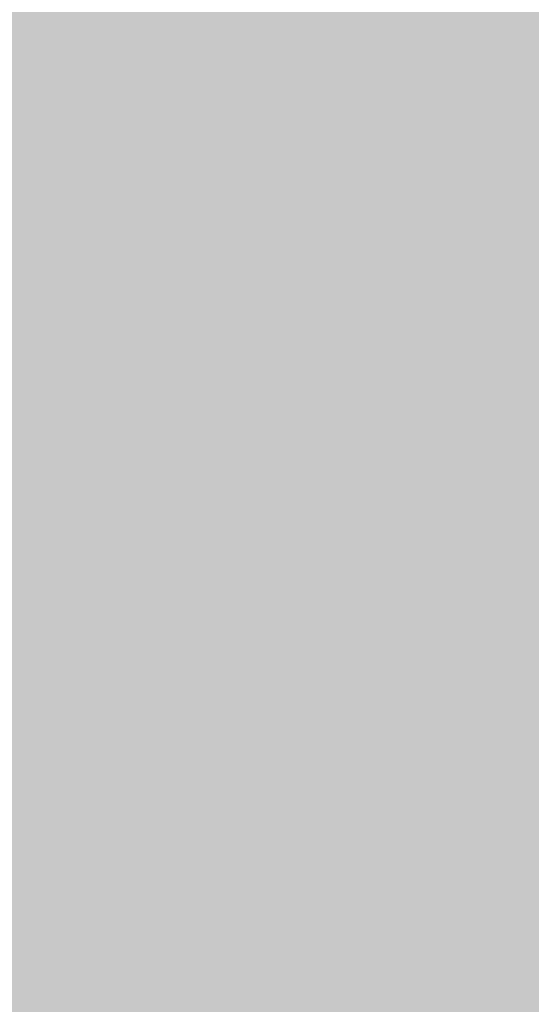
# Model space of a CAD drawing. Units: inches. Extents: x 2083 to 3317, y 1141 to 2115.
# Tile 206 of 256: x 3126.132 to 3126.67, y 1264.131 to 1265.165. Entities that reach past the tile are written whole.
import ezdxf

# ---------------------------------------------------------------- set-up
doc = ezdxf.new("R2010")
doc.units = ezdxf.units.IN
doc.layers.add('A-ANNO-DIMS', color=2, linetype='Continuous', lineweight=18)
doc.layers.add('A-WALL-PATT', color=251, linetype='Continuous', lineweight=13, true_color=0x636466)
doc.styles.get("Standard").update_dxf_attribs({"font": 'arial.ttf'})
doc.dimstyles.new('ISO-25', dxfattribs={"dimtxt": 12, "dimasz": 12, "dimexe": 1.25, "dimexo": 0.625, "dimtad": 1, "dimlunit": 3, "dimtxsty": 'Standard', "dimcen": 2.5, "dimadec": 0, "dimazin": 0, "dimtfac": 1, "dimtmove": 0, "dimatfit": 3, "dimfxl": 1, "dimarcsym": 0})

# ---------------------------------------------------------------- blocks, each defined once
blk = doc.blocks.new('*D26')
at = {"layer": 'A-ANNO-DIMS', "color": 0, "lineweight": -2, "transparency": 16777216}
for p, q in [((3088.9858, 1274.9151), (3088.9858, 1270.952)), ((3111.24, 1274.9151), (3111.24, 1270.952)), ((3076.9858, 1272.202), (2840.2624, 1272.202)), ((3111.24, 1272.202), (3088.9858, 1272.202)), ((3123.24, 1272.202), (3135.24, 1272.202))]:
    blk.add_line(p, q, dxfattribs=at)
at = {"layer": 'A-ANNO-DIMS', "color": 0, "transparency": 16777216}
for points in [[(3076.9858, 1274.202), (3076.9858, 1270.202), (3088.9858, 1272.202)], [(3123.24, 1274.202), (3123.24, 1270.202), (3111.24, 1272.202)]]:
    blk.add_solid(points, dxfattribs=at)
at = {"layer": 'Defpoints', "color": 0, "transparency": 16777216}
for p in [(3088.9858, 1275.5401), (3111.24, 1275.5401), (3088.9858, 1272.202)]:
    blk.add_point(p, dxfattribs=at)
at = {"layer": 'A-ANNO-DIMS', "color": 0, "transparency": 16777216, "insert": (2952.6241, 1279.0316), "char_height": 12, "attachment_point": 5}
blk.add_mtext('NIGHTSTAND 1\'-10 1/2" TYP.', dxfattribs=at)
blk = doc.blocks.new('*D27')
at = {"layer": 'A-ANNO-DIMS', "color": 0, "lineweight": -2, "transparency": 16777216}
for p, q in [((3114.5782, 1309.7943), (3114.5782, 1321.7943)), ((3111.865, 1297.7943), (3115.8282, 1297.7943)), ((3114.5782, 1297.7943), (3114.5782, 1275.5401)), ((3111.865, 1275.5401), (3115.8282, 1275.5401)), ((3114.5782, 1263.5401), (3114.5782, 1140.9886))]:
    blk.add_line(p, q, dxfattribs=at)
at = {"layer": 'A-ANNO-DIMS', "color": 0, "transparency": 16777216}
for points in [[(3112.5782, 1309.7943), (3116.5782, 1309.7943), (3114.5782, 1297.7943)], [(3112.5782, 1263.5401), (3116.5782, 1263.5401), (3114.5782, 1275.5401)]]:
    blk.add_solid(points, dxfattribs=at)
at = {"layer": 'Defpoints', "color": 0, "transparency": 16777216}
for p in [(3111.24, 1297.7943), (3111.24, 1275.5401), (3114.5782, 1275.5401)]:
    blk.add_point(p, dxfattribs=at)
at = {"layer": 'A-ANNO-DIMS', "color": 0, "transparency": 16777216, "insert": (3107.7485, 1196.2643), "char_height": 12, "attachment_point": 5, "rotation": 90}
blk.add_mtext('1\'-10 1/2" TYP.', dxfattribs=at)

msp = doc.modelspace()

# ---------------------------------------------------------------- hatches: boundary and pattern name
at = {"layer": 'A-WALL-PATT'}
h = msp.add_hatch(color=256, dxfattribs=at)
h.dxf.hatch_style = 1
h.paths.add_polyline_path([(3126.9598, 2020.7614), (2748.9598, 2020.7614), (2604.9598, 2020.7614), (2226.9598, 2020.7614), (2226.9598, 1702.7614), (2466.9598, 1702.7614), (2466.9598, 1582.7614), (2418.9598, 1582.7614), (2418.9598, 1477.7614), (2226.9598, 1477.7614), (2226.9598, 1263.2614), (2544.9598, 1263.2614), (2544.9598, 1411.7614), (2604.9598, 1411.7614), (2685.9598, 1411.7614), (2685.9598, 1420.7614), (2604.9598, 1420.7614), (2604.9598, 1573.7614), (2604.9598, 1702.7614), (2604.9598, 2011.7614), (2748.9598, 2011.7614), (2748.9598, 1702.7614), (2862.9598, 1702.7614), (2862.9598, 1621.7614), (2871.9598, 1621.7614), (2871.9598, 1702.7614), (2883.9598, 1702.7614), (2883.9598, 1706.9395, -0.026459), (2883.9598, 1711.7614), (2757.9598, 1711.7614), (2757.9598, 1807.7614), (2787.9598, 1807.7614), (2787.9598, 1812.2614), (2757.9598, 1812.2614), (2757.9598, 2011.7614), (2877.9598, 2011.7614), (2877.9598, 1812.2614), (2847.9598, 1812.2614), (2847.9598, 1807.7614), (2889.8357, 1807.7614), (2889.8357, 1812.2614), (2882.4598, 1812.2614), (2882.4598, 2011.7614), (3117.9598, 2011.7614), (3117.9598, 1812.2614), (2937.8357, 1812.2614), (2937.8357, 1807.7614), (2995.7098, 1807.7614), (2995.7098, 1796.1177), (3000.2098, 1796.1177), (3000.2098, 1807.7614), (3117.9598, 1807.7614), (3117.9598, 1711.7614), (3000.2098, 1711.7614), (3000.2098, 1760.1177), (2998.5727, 1760.1177, -0.020711), (2995.7098, 1760.1177), (2995.7098, 1711.7614), (2931.9598, 1711.7614), (2931.9598, 1702.7614), (3126.9598, 1702.7614)])
h.paths.add_polyline_path([(2471.4598, 2011.7614), (2471.4598, 1810.0114), (2462.7169, 1810.0114), (2462.7169, 1805.5114), (2505.9598, 1805.5114), (2505.9598, 1810.0114), (2475.9598, 1810.0114), (2475.9598, 2011.7614), (2595.9598, 2011.7614), (2595.9598, 1810.0114), (2565.9598, 1810.0114), (2565.9598, 1805.5114), (2595.9598, 1805.5114), (2595.9598, 1711.7614), (2235.9598, 1711.7614), (2235.9598, 1805.5114), (2353.7098, 1805.5114), (2353.7098, 1796.0542), (2358.2098, 1796.0542), (2358.2098, 1805.5114), (2414.7169, 1805.5114), (2414.7169, 1810.0114), (2235.9598, 1810.0114), (2235.9598, 2011.7614)], flags=16)
h.paths.add_polyline_path([(2270.2047, 1994.61), (2270.2047, 1970.61), (2246.2047, 1970.61), (2246.2047, 1994.61)], flags=0)
edge = h.paths.add_edge_path(flags=0)
edge.add_ellipse((2332.0274, 1899.7982), major_axis=(-3.043, 3.043), ratio=0.168252, start_angle=-161.3322, end_angle=-156.3071, ccw=False)
edge.add_ellipse((2333.082, 1898.7435), major_axis=(-1.0546, 1.0546), ratio=0.453532, start_angle=-123.371, end_angle=-94.1591)
edge = h.paths.add_edge_path(flags=0)
edge.add_ellipse((2332.0274, 1968.8763), major_axis=(3.043, 3.043), ratio=0.168252, start_angle=18.6678, end_angle=23.6929)
edge.add_spline(control_points=[(2332.9256, 1970.6911), (2332.2268, 1970.3361), (2330.8937, 1969.6589), (2328.4131, 1970.9321), (2327.2039, 1967.7487), (2324.7096, 1969.9556), (2322.5328, 1967.0124), (2320.0128, 1971.2958), (2317.6803, 1968.1578), (2316.0405, 1967.102), (2315.4269, 1966.8096)], knot_values=[0, 0, 0, 0, 2.267059, 4.324559, 6.685584, 8.878641, 11.121502, 14.300359, 17.755284, 19.732645, 19.732645, 19.732645, 19.732645], degree=3, periodic=0)
edge.add_ellipse((2332.0274, 1968.8763), major_axis=(3.043, 3.043), ratio=0.168252, start_angle=18.6678, end_angle=23.6929, ccw=False)
edge.add_ellipse((2333.082, 1969.9309), major_axis=(1.0546, 1.0546), ratio=0.453532, start_angle=56.629, end_angle=85.8409, ccw=False)
edge = h.paths.add_edge_path(flags=0)
edge.add_spline(control_points=[(2296.4283, 1967.9879), (2293.6278, 1965.3363), (2287.7036, 1959.7271), (2299.7439, 1949.9957), (2294.5326, 1935.6685), (2290.5732, 1920.6035), (2293.3941, 1909.9737), (2296.1854, 1904.9665)], knot_values=[0.099185, 0.099185, 0.099185, 0.099185, 0.345301, 0.619822, 0.982653, 1.386093, 1.810555, 1.810555, 1.810555, 1.810555], degree=3, periodic=0)
edge.add_spline(control_points=[(2296.1854, 1904.9665), (2297.3836, 1902.6193), (2298.001, 1901.9493), (2298.553, 1901.4682)], knot_values=[0.006246, 0.006246, 0.006246, 0.006246, 0.055476, 0.055476, 0.055476, 0.055476], degree=3, periodic=0)
edge.add_spline(control_points=[(2298.553, 1901.4682), (2297.2586, 1900.9232), (2295.2253, 1900.2321), (2293.0602, 1900.6142), (2292.1014, 1900.7884), (2292.0896, 1900.7906)], knot_values=[0.312835, 0.312835, 0.312835, 0.312835, 0.40178, 0.474987, 0.475903, 0.475903, 0.475903, 0.475903], degree=3, periodic=0)
edge.add_arc((2292.7936, 1904.6641), 3.937, 215.4209, 259.6982, ccw=False)
edge.add_spline(control_points=[(2289.5853, 1902.3823), (2289.4767, 1902.5351), (2289.3685, 1902.688), (2289.2609, 1902.8412)], knot_values=[0.102872, 0.102872, 0.102872, 0.102872, 0.116896, 0.116896, 0.116896, 0.116896], degree=3, periodic=0)
edge.add_spline(control_points=[(2289.2609, 1902.8412), (2288.6866, 1902.5502), (2287.64, 1902.0199), (2285.8813, 1901.874), (2283.853, 1901.5044), (2281.72, 1899.7105), (2278.467, 1899.4929), (2276.1571, 1901.8832), (2272.259, 1899.8041), (2267.7776, 1901.8432), (2262.2439, 1900.184), (2257.4149, 1901.7821), (2254.3184, 1900.7261), (2253.1783, 1900.3373)], knot_values=[0, 0, 0, 0, 1.907977, 3.477176, 5.261074, 7.972851, 11.680248, 13.717921, 16.939592, 22.789562, 27.502503, 33.595215, 37.145618, 37.145618, 37.145618, 37.145618], degree=3, periodic=0)
edge.add_line((2253.1783, 1900.3373), (2250.2442, 1902.8412))
edge.add_line((2250.2442, 1902.8412), (2250.2442, 1965.8333))
edge.add_line((2250.2442, 1965.8333), (2253.1783, 1968.3371))
edge.add_spline(control_points=[(2253.1783, 1968.3371), (2254.3184, 1967.9483), (2257.4149, 1966.8924), (2262.2439, 1968.4904), (2267.7776, 1966.8313), (2271.5267, 1968.5372), (2273.8759, 1967.8283), (2274.2067, 1967.7276)], knot_values=[0, 0, 0, 0, 0.09018, 0.244935, 0.364644, 0.513233, 0.537855, 0.537855, 0.537855, 0.537855], degree=3, periodic=0)
edge.add_arc((2274.3529, 1963.7933), 3.937, 72.0511, 92.1279, ccw=False)
edge.add_arc((2281.2969, 1985.23), 18.5963, 252.05113, 288.56572)
edge.add_arc((2292.3167, 1956.0289), 12.6461, 71.02679, 113.77822, ccw=False)
edge = h.paths.add_edge_path(flags=0)
edge.add_spline(control_points=[(2274.8994, 1951.8562), (2275.0662, 1951.6166), (2275.2327, 1951.3766), (2275.398, 1951.1359)], knot_values=[1.409916, 1.409916, 1.409916, 1.409916, 1.43159, 1.43159, 1.43159, 1.43159], degree=3, periodic=0)
edge.add_spline(control_points=[(2275.398, 1951.1359), (2275.7921, 1950.5619), (2276.1792, 1949.9838), (2276.5455, 1949.3971)], knot_values=[1.358238, 1.358238, 1.358238, 1.358238, 1.409916, 1.409916, 1.409916, 1.409916], degree=3, periodic=0)
edge.add_line((2276.5455, 1949.3971), (2277.4373, 1947.8622))
edge.add_spline(control_points=[(2277.4373, 1947.8622), (2276.3038, 1945.6731), (2274.6397, 1942.4269), (2274.6316, 1938.0939), (2272.7991, 1930.8515), (2274.3564, 1943.897), (2275.9477, 1947.9234), (2276.5455, 1949.3971)], knot_values=[0.005632, 0.005632, 0.005632, 0.005632, 0.186014, 0.266002, 0.357087, 0.59639, 0.739732, 0.739732, 0.739732, 0.739732], degree=3, periodic=0)
edge.add_spline(control_points=[(2276.5455, 1949.3971), (2276.1792, 1949.9838), (2275.7921, 1950.5619), (2275.398, 1951.1359)], knot_values=[1.358238, 1.358238, 1.358238, 1.358238, 1.409916, 1.409916, 1.409916, 1.409916], degree=3, periodic=0)
edge.add_spline(control_points=[(2275.398, 1951.1359), (2274.9425, 1950.0805), (2274.2078, 1948.0253), (2273.9346, 1944.8515), (2272.4685, 1937.6275), (2273.4662, 1945.6965), (2274.7006, 1951.0595), (2274.8994, 1951.8562)], knot_values=[0.104364, 0.104364, 0.104364, 0.104364, 0.189636, 0.269624, 0.36071, 0.600013, 0.644622, 0.644622, 0.644622, 0.644622], degree=3, periodic=0)
h.paths.add_polyline_path([(2269.1675, 1963.1276, -0.357527), (2268.1706, 1960.9764, -0.092561), (2268.1706, 1939.4363, -0.357527), (2269.1675, 1937.2851, -0.357527), (2267.0163, 1938.282, -0.164785), (2254.6856, 1938.282, -0.357527), (2252.5344, 1937.2851, -0.357527), (2253.5313, 1939.4363, -0.092561), (2253.5313, 1960.9764, -0.357527), (2252.5344, 1963.1276, -0.357527), (2254.6856, 1962.1307, -0.164785), (2267.0163, 1962.1307, -0.357527)], flags=0)
h.paths.add_polyline_path([(2248.8741, 1967.8018), (2248.8741, 1957.0277), (2249.4578, 1957.0277), (2249.4578, 1911.6468), (2248.8741, 1911.6468), (2248.8741, 1900.8727), (2246.5119, 1900.8727, 0.197327), (2244.1497, 1902.4569), (2244.1497, 1966.2176, 0.197327), (2246.5119, 1967.8018)], flags=0)
h.paths.add_polyline_path([(2269.1675, 1931.3893, -0.357527), (2268.1706, 1929.2381, -0.092561), (2268.1706, 1907.6981, -0.357527), (2269.1675, 1905.5469, -0.357527), (2267.0163, 1906.5438, -0.164785), (2254.6856, 1906.5438, -0.357527), (2252.5344, 1905.5469, -0.357527), (2253.5313, 1907.6981, -0.092561), (2253.5313, 1929.2381, -0.357527), (2252.5344, 1931.3893, -0.357527), (2254.6856, 1930.3925, -0.164785), (2267.0163, 1930.3925, -0.357527)], flags=0)
edge = h.paths.add_edge_path(flags=0)
edge.add_spline(control_points=[(2276.1969, 1906.7237), (2276.1681, 1909.0289), (2276.114, 1913.3719), (2270.5984, 1924.925), (2273.9052, 1919.0128), (2275.9217, 1916.2621), (2275.4746, 1912.4021), (2277.2579, 1910.3806), (2276.696, 1908.225), (2276.6462, 1906.813), (2276.6178, 1906.0084)], knot_values=[0, 0, 0, 0, 8.61026, 16.221274, 18.843057, 23.804898, 27.440828, 29.356102, 31.203478, 33.650687, 33.650687, 33.650687, 33.650687], degree=3, periodic=0)
edge.add_spline(control_points=[(2276.6178, 1906.0084), (2276.6233, 1905.6241), (2276.4977, 1904.6287), (2275.4418, 1903.8547), (2274.9373, 1903.0804), (2274.8591, 1902.8412)], knot_values=[0.156488, 0.156488, 0.156488, 0.156488, 0.184398, 0.231376, 0.250598, 0.250598, 0.250598, 0.250598], degree=3, periodic=0)
edge.add_line((2274.8591, 1902.8412), (2276.506, 1902.8412))
edge.add_spline(control_points=[(2276.506, 1902.8412), (2276.7883, 1903.0849), (2277.6651, 1904.1252), (2278.2495, 1904.3407), (2277.6539, 1908.5274), (2278.1557, 1906.2278), (2278.1005, 1905.2859), (2278.8467, 1904.069), (2277.8568, 1903.4149), (2277.8742, 1902.991), (2277.9036, 1902.8412)], knot_values=[0.059574, 0.059574, 0.059574, 0.059574, 0.080753, 0.103741, 0.16972, 0.176036, 0.207137, 0.240474, 0.262341, 0.27366, 0.27366, 0.27366, 0.27366], degree=3, periodic=0)
edge.add_line((2277.9036, 1902.8412), (2280.0298, 1902.8412))
edge.add_spline(control_points=[(2280.0298, 1902.8412), (2279.8882, 1903.0884), (2279.4993, 1903.9816), (2280.1523, 1905.9393), (2278.1036, 1909.6578), (2279.7624, 1907.1853), (2280.3279, 1904.8749), (2280.4851, 1903.4896), (2281.4633, 1903.2494), (2281.7583, 1902.9365), (2281.834, 1902.8412)], knot_values=[0.013856, 0.013856, 0.013856, 0.013856, 0.034874, 0.088867, 0.107879, 0.126738, 0.158714, 0.193757, 0.217487, 0.226722, 0.226722, 0.226722, 0.226722], degree=3, periodic=0)
edge.add_spline(control_points=[(2281.834, 1902.8412), (2281.7875, 1902.8267), (2281.647, 1902.783), (2281.3955, 1902.8595), (2281.0881, 1902.9852), (2280.7207, 1903.0609), (2280.3335, 1903.0257), (2280.1248, 1902.8989), (2280.0298, 1902.8412)], knot_values=[0, 0, 0, 0, 0.14413, 0.435517, 0.749276, 1.153046, 1.548371, 1.878348, 1.878348, 1.878348, 1.878348], degree=3, periodic=0)
edge.add_line((2280.0298, 1902.8412), (2277.9036, 1902.8412))
edge.add_spline(control_points=[(2277.9036, 1902.8412), (2277.8929, 1902.7959), (2277.8654, 1902.6796), (2277.6075, 1902.6875), (2277.2741, 1902.8007), (2276.8379, 1902.6198), (2276.5838, 1902.7893), (2276.506, 1902.8412)], knot_values=[0, 0, 0, 0, 0.127189, 0.326199, 0.628009, 1.24357, 1.515331, 1.515331, 1.515331, 1.515331], degree=3, periodic=0)
edge.add_line((2276.506, 1902.8412), (2274.8591, 1902.8412))
edge.add_spline(control_points=[(2274.8591, 1902.8412), (2274.8144, 1902.8986), (2274.7251, 1903.0134), (2274.4935, 1903.119), (2274.2443, 1902.9605), (2273.9371, 1903.1849), (2273.614, 1902.9831), (2273.4083, 1902.883), (2273.3223, 1902.8412)], knot_values=[0, 0, 0, 0, 0.21843, 0.436957, 0.687977, 0.990379, 1.398396, 1.69185, 1.69185, 1.69185, 1.69185], degree=3, periodic=0)
edge.add_spline(control_points=[(2273.3223, 1902.8412), (2273.6167, 1903.4457), (2274.274, 1904.5383), (2276.0272, 1904.5737), (2276.207, 1906.5836), (2276.1969, 1906.7237)], knot_values=[0.012227, 0.012227, 0.012227, 0.012227, 0.059472, 0.106218, 0.134458, 0.134458, 0.134458, 0.134458], degree=3, periodic=0)
h.paths.add_polyline_path([(2270.7761, 1897.7898), (2270.7761, 1873.7898), (2246.7761, 1873.7898), (2246.7761, 1897.7898)], flags=0)
h.paths.add_polyline_path([(2353.7098, 1760.0051), (2353.7098, 1760.0542), (2358.2098, 1760.0542, -0.033729)], flags=0)
h.paths.add_polyline_path([(2321.8191, 1737.5292), (2341.9953, 1737.5292, -0.414214), (2343.2033, 1736.3212), (2343.2033, 1721.0206, -0.414214), (2341.9953, 1719.8127), (2321.8191, 1719.8127, -0.414214), (2320.6112, 1721.0206), (2320.6112, 1736.3212, -0.414214)], flags=0)
h.paths.add_polyline_path([(2324.235, 1736.3212), (2339.5794, 1736.3212, -0.414214), (2341.9953, 1733.9053), (2341.9953, 1725.4497, -0.414214), (2339.5794, 1723.0338), (2333.6806, 1723.0338), (2333.8453, 1722.0455, -0.870646), (2335.4254, 1721.8259, -0.767327), (2333.9227, 1721.4232), (2331.291, 1721.4232, -0.767327), (2329.7883, 1721.8259, -0.870646), (2331.3684, 1722.0455), (2331.5331, 1723.0338), (2324.235, 1723.0338, -0.414214), (2321.8191, 1725.4497), (2321.8191, 1733.9053, -0.414214)], flags=0)
h.paths.add_polyline_path([(2570.4838, 1928.6154), (2589.6838, 1928.6154), (2590.1688, 1928.6154), (2590.1688, 1904.9934), (2570.4838, 1904.9934)], flags=0)
h.paths.add_polyline_path([(2574.4473, 1927.2638, -1), (2572.8288, 1927.2638, -1)], flags=0)
h.paths.add_polyline_path([(2573.0899, 1926.9409), (2573.925, 1927.776), (2574.1477, 1927.5533), (2573.3126, 1926.7182)], flags=0)
h.paths.add_polyline_path([(2578.7791, 1919.7296, -1), (2571.5917, 1919.7296, -1)], flags=0)
h.paths.add_polyline_path([(2578.3854, 1919.7296, -1), (2571.9854, 1919.7296, -1)], flags=0)
h.paths.add_polyline_path([(2331.5958, 1729.4762, -1), (2333.618, 1729.4762, -1)], flags=0)
h.paths.add_polyline_path([(2578.0342, 1927.2638, -1), (2576.4157, 1927.2638, -1)], flags=0)
h.paths.add_polyline_path([(2576.6889, 1927.5311), (2576.9116, 1927.7538), (2577.7467, 1926.9186), (2577.524, 1926.6959)], flags=0)
h.paths.add_polyline_path([(2578.1391, 1909.8595, -1), (2572.2317, 1909.8595, -1)], flags=0)
h.paths.add_polyline_path([(2577.7454, 1909.8595, -1), (2572.6254, 1909.8595, -1)], flags=0)
h.paths.add_polyline_path([(2583.7977, 1927.2638, -1), (2582.1792, 1927.2638, -1)], flags=0)
h.paths.add_polyline_path([(2582.7186, 1927.7538), (2583.5538, 1926.9186), (2583.3311, 1926.6959), (2582.4959, 1927.5311)], flags=0)
h.paths.add_polyline_path([(2582.4959, 1927.5311), (2582.7186, 1927.7538), (2583.5538, 1926.9186), (2583.3311, 1926.6959)], flags=0)
h.paths.add_polyline_path([(2587.7391, 1920.5296, -1), (2581.8317, 1920.5296, -1)], flags=0)
h.paths.add_polyline_path([(2587.3454, 1920.5296, -1), (2582.2254, 1920.5296, -1)], flags=0)
h.paths.add_polyline_path([(2587.3846, 1927.2638, -1), (2585.7661, 1927.2638, -1)], flags=0)
h.paths.add_polyline_path([(2586.082, 1926.9802), (2586.9172, 1927.8154), (2587.1399, 1927.5927), (2586.3047, 1926.7575)], flags=0)
h.paths.add_polyline_path([(2588.3791, 1910.6595, -1), (2581.1917, 1910.6595, -1)], flags=0)
h.paths.add_polyline_path([(2587.9854, 1910.6595, -1), (2581.5854, 1910.6595, -1)], flags=0)
h.paths.add_polyline_path([(2417.1677, 1729.4779), (2437.3439, 1729.4779, -0.414214), (2438.5519, 1728.2699), (2438.5519, 1712.9693, -0.414214), (2437.3439, 1711.7614), (2417.1677, 1711.7614, -0.414214), (2415.9598, 1712.9693), (2415.9598, 1728.2699, -0.414214)], flags=0)
h.paths.add_polyline_path([(2419.5836, 1728.2699), (2434.928, 1728.2699, -0.414214), (2437.3439, 1725.8541), (2437.3439, 1717.3984, -0.414214), (2434.928, 1714.9825), (2429.0292, 1714.9825), (2429.1939, 1713.9942, -0.870646), (2430.774, 1713.7746, -0.767327), (2429.2713, 1713.372), (2426.6396, 1713.372, -0.767327), (2425.1369, 1713.7746, -0.870646), (2426.717, 1713.9942), (2426.8817, 1714.9825), (2419.5836, 1714.9825, -0.414214), (2417.1677, 1717.3984), (2417.1677, 1725.8541, -0.414214)], flags=0)
h.paths.add_polyline_path([(2419.5836, 1728.2699), (2434.928, 1728.2699, -0.414214), (2437.3439, 1725.8541), (2437.3439, 1717.3984, -0.414214), (2434.928, 1714.9825), (2429.0292, 1714.9825), (2428.3581, 1719.009), (2427.5528, 1719.009), (2426.8817, 1714.9825), (2419.5836, 1714.9825, -0.414214), (2417.1677, 1717.3984), (2417.1677, 1725.8541, -0.414214)], flags=0)
h.paths.add_polyline_path([(2426.9444, 1721.4249, -1), (2428.9666, 1721.4249, -1)], flags=0)
h.paths.add_polyline_path([(2475.9598, 1702.7614), (2595.9598, 1702.7614), (2595.9598, 1582.7614), (2475.9598, 1582.7614)], flags=16)
h.paths.add_polyline_path([(2427.9598, 1573.7614), (2595.9598, 1573.7614), (2595.9598, 1468.7614), (2595.9598, 1420.7614), (2384.4598, 1420.7614), (2384.4598, 1468.7614), (2427.9598, 1468.7614)], flags=16)
h.paths.add_polyline_path([(2379.9598, 1468.7614), (2379.9598, 1420.7614), (2235.9598, 1420.7614), (2235.9598, 1468.7614)], flags=16)
h.paths.add_polyline_path([(2317.816, 1466.6958), (2337.9922, 1466.6958, -0.414214), (2339.2002, 1465.4878), (2339.2002, 1450.1872, -0.414214), (2337.9922, 1448.9792), (2317.816, 1448.9792, -0.414214), (2316.6081, 1450.1872), (2316.6081, 1465.4878, -0.414214)], flags=0)
h.paths.add_polyline_path([(2320.2319, 1465.4878), (2335.5763, 1465.4878, -0.414214), (2337.9922, 1463.0719), (2337.9922, 1454.6163, -0.414214), (2335.5763, 1452.2004), (2329.6775, 1452.2004), (2329.8422, 1451.212, -0.870646), (2331.4223, 1450.9925, -0.767327), (2329.9196, 1450.5898), (2327.2879, 1450.5898, -0.767327), (2325.7852, 1450.9925, -0.870646), (2327.3653, 1451.212), (2327.53, 1452.2004), (2320.2319, 1452.2004, -0.414214), (2317.816, 1454.6163), (2317.816, 1463.0719, -0.414214)], flags=0)
h.paths.add_polyline_path([(2320.2319, 1465.4878), (2335.5763, 1465.4878, -0.414214), (2337.9922, 1463.0719), (2337.9922, 1454.6163, -0.414214), (2335.5763, 1452.2004), (2329.6775, 1452.2004), (2329.0064, 1456.2269), (2328.2011, 1456.2269), (2327.53, 1452.2004), (2320.2319, 1452.2004, -0.414214), (2317.816, 1454.6163), (2317.816, 1463.0719, -0.414214)], flags=0)
h.paths.add_polyline_path([(2327.5926, 1458.6428, -1), (2329.6148, 1458.6428, -1)], flags=0)
h.paths.add_polyline_path([(2244.4117, 1433.3405), (2241.9209, 1433.3405, -0.414214), (2240.0179, 1435.2435), (2240.0179, 1440.9528, -0.414211), (2241.9209, 1442.8559), (2244.4117, 1442.8559, -1.976472)], flags=0)
h.paths.add_polyline_path([(2245.3569, 1434.3975, -0.414214), (2245.3569, 1441.7988, -2.144098)], flags=0)
h.paths.add_polyline_path([(2535.9598, 1416.2614), (2535.9598, 1272.2614), (2235.9598, 1272.2614), (2235.9598, 1416.2614)], flags=16)
h.paths.add_polyline_path([(2260.1196, 1384.2928), (2260.1196, 1362.0386), (2237.8654, 1362.0386), (2237.8654, 1384.2928)], flags=0)
edge = h.paths.add_edge_path(flags=0)
edge.add_line((2318.2518, 1362.0933), (2318.1458, 1362.001))
edge.add_ellipse((2317.4451, 1360.431), major_axis=(2.8216, 2.8216), ratio=0.168252, start_angle=18.6678, end_angle=20.9481, ccw=False)
edge.add_ellipse((2318.423, 1361.409), major_axis=(0.9779, 0.9779), ratio=0.453532, start_angle=56.629, end_angle=70.2262, ccw=False)
edge = h.paths.add_edge_path(flags=0)
edge.add_line((2319.1074, 1295.5711), (2319.015, 1295.6771))
edge.add_ellipse((2317.4451, 1296.3778), major_axis=(-2.8216, 2.8216), ratio=0.168252, start_angle=-161.3322, end_angle=-159.0519, ccw=False)
edge.add_ellipse((2318.423, 1295.3999), major_axis=(-0.9779, 0.9779), ratio=0.453532, start_angle=-123.371, end_angle=-109.7738)
edge = h.paths.add_edge_path(flags=0)
edge.add_spline(control_points=[(2284.2103, 1301.1702), (2284.5807, 1300.4447), (2284.8912, 1299.892), (2285.1596, 1299.461)], knot_values=[0.039066, 0.039066, 0.039066, 0.039066, 0.055476, 0.055476, 0.055476, 0.055476], degree=3, periodic=0)
edge.add_line((2285.1596, 1299.461), (2284.2103, 1301.1702))
edge = h.paths.add_edge_path(flags=0)
edge.add_line((2280.4125, 1297.298), (2283.37, 1297.0361))
edge.add_line((2283.37, 1297.0361), (2286.4057, 1297.9263))
edge.add_spline(control_points=[(2286.4057, 1297.9263), (2285.3055, 1297.4631), (2284.3448, 1297.1292), (2283.37, 1297.0361)], knot_values=[0.394369, 0.394369, 0.394369, 0.394369, 0.475903, 0.475903, 0.475903, 0.475903], degree=3, periodic=0)
edge.add_spline(control_points=[(2283.37, 1297.0361), (2283.2814, 1297.0277), (2282.3163, 1296.9573), (2281.3125, 1297.1345), (2280.4234, 1297.296), (2280.4125, 1297.298)], knot_values=[0.312835, 0.312835, 0.312835, 0.312835, 0.320246, 0.393453, 0.394369, 0.394369, 0.394369, 0.394369], degree=3, periodic=0)
edge = h.paths.add_edge_path(flags=0)
edge.add_line((2284.4356, 1359.6073), (2280.4463, 1355.328))
edge.add_line((2280.4463, 1355.328), (2279.58, 1351.0178))
edge.add_line((2279.58, 1351.0178), (2282.413, 1346.5804))
edge.add_spline(control_points=[(2282.413, 1346.5804), (2283.1533, 1345.5892), (2284.2529, 1344.0289), (2284.801, 1342.3872), (2284.9352, 1341.8055)], knot_values=[1.240098, 1.240098, 1.240098, 1.240098, 1.332892, 1.382712, 1.382712, 1.382712, 1.382712], degree=3, periodic=0)
edge.add_spline(control_points=[(2284.9352, 1341.8055), (2285.3191, 1340.1406), (2285.233, 1338.4092), (2284.9099, 1336.6541)], knot_values=[1.097484, 1.097484, 1.097484, 1.097484, 1.240098, 1.240098, 1.240098, 1.240098], degree=3, periodic=0)
edge.add_spline(control_points=[(2284.9099, 1336.6541), (2284.5868, 1334.899), (2284.0267, 1333.1203), (2283.4626, 1331.3606)], knot_values=[0.95487, 0.95487, 0.95487, 0.95487, 1.097484, 1.097484, 1.097484, 1.097484], degree=3, periodic=0)
edge.add_line((2283.4626, 1331.3606), (2281.8904, 1326.1534))
edge.add_line((2281.8904, 1326.1534), (2280.7563, 1321.0561))
edge.add_line((2280.7563, 1321.0561), (2280.2992, 1316.002))
edge.add_line((2280.2992, 1316.002), (2280.7159, 1310.9501))
edge.add_line((2280.7159, 1310.9501), (2282.0281, 1305.9721))
edge.add_line((2282.0281, 1305.9721), (2284.2103, 1301.1702))
edge.add_spline(control_points=[(2284.2103, 1301.1702), (2283.3407, 1302.7302), (2282.6119, 1304.3365), (2282.0281, 1305.9721)], knot_values=[0.099185, 0.099185, 0.099185, 0.099185, 0.241799, 0.241799, 0.241799, 0.241799], degree=3, periodic=0)
edge.add_spline(control_points=[(2282.0281, 1305.9721), (2281.4443, 1307.6078), (2281.0055, 1309.2728), (2280.7159, 1310.9501)], knot_values=[0.241799, 0.241799, 0.241799, 0.241799, 0.384413, 0.384413, 0.384413, 0.384413], degree=3, periodic=0)
edge.add_spline(control_points=[(2280.7159, 1310.9501), (2280.4332, 1312.5876), (2280.2894, 1314.277), (2280.2989, 1315.962), (2280.2992, 1316.002)], knot_values=[0.384413, 0.384413, 0.384413, 0.384413, 0.523647, 0.527028, 0.527028, 0.527028, 0.527028], degree=3, periodic=0)
edge.add_spline(control_points=[(2280.2992, 1316.002), (2280.3123, 1317.687), (2280.4779, 1319.3679), (2280.7563, 1321.0561)], knot_values=[0.527028, 0.527028, 0.527028, 0.527028, 0.669642, 0.669642, 0.669642, 0.669642], degree=3, periodic=0)
edge.add_spline(control_points=[(2280.7563, 1321.0561), (2281.0346, 1322.7443), (2281.4259, 1324.4396), (2281.8904, 1326.1534)], knot_values=[0.669642, 0.669642, 0.669642, 0.669642, 0.812256, 0.812256, 0.812256, 0.812256], degree=3, periodic=0)
edge.add_spline(control_points=[(2281.8904, 1326.1534), (2282.2644, 1327.5333), (2282.7879, 1329.2618), (2283.3528, 1331.0178), (2283.4626, 1331.3606)], knot_values=[0.812256, 0.812256, 0.812256, 0.812256, 0.927087, 0.95487, 0.95487, 0.95487, 0.95487], degree=3, periodic=0)
edge.add_line((2283.4626, 1331.3606), (2284.9099, 1336.6541))
edge.add_line((2284.9099, 1336.6541), (2284.9352, 1341.8055))
edge.add_line((2284.9352, 1341.8055), (2282.413, 1346.5804))
edge.add_spline(control_points=[(2282.413, 1346.5804), (2281.2751, 1348.1038), (2280.0784, 1349.5703), (2279.58, 1351.0178)], knot_values=[1.382712, 1.382712, 1.382712, 1.382712, 1.525326, 1.525326, 1.525326, 1.525326], degree=3, periodic=0)
edge.add_spline(control_points=[(2279.58, 1351.0178), (2279.4433, 1351.4147), (2279.1363, 1352.8569), (2279.7352, 1354.2904), (2280.4463, 1355.328)], knot_values=[1.525326, 1.525326, 1.525326, 1.525326, 1.564439, 1.667941, 1.667941, 1.667941, 1.667941], degree=3, periodic=0)
edge.add_spline(control_points=[(2280.4463, 1355.328), (2281.4261, 1356.7578), (2282.9308, 1358.1826), (2284.4356, 1359.6073)], knot_values=[1.667941, 1.667941, 1.667941, 1.667941, 1.810555, 1.810555, 1.810555, 1.810555], degree=3, periodic=0)
edge.add_arc((2280.6231, 1348.5182), 11.7262, 71.02679, 113.77822)
edge.add_arc((2270.4049, 1375.5952), 17.2436, 252.05113, 288.56572, ccw=False)
edge.add_arc((2263.966, 1355.7178), 3.6506, 72.0511, 92.1279)
edge.add_arc((2263.966, 1355.7178), 3.6506, 92.1279, 177.9851)
edge.add_spline(control_points=[(2260.3176, 1355.8462), (2260.2604, 1354.2207), (2260.5513, 1350.1865), (2262.9993, 1346.7663), (2264.4727, 1344.649)], knot_values=[1.43159, 1.43159, 1.43159, 1.43159, 1.564144, 1.770695, 1.770695, 1.770695, 1.770695], degree=3, periodic=0)
edge.add_line((2264.4727, 1344.649), (2264.9356, 1343.9825))
edge.add_spline(control_points=[(2263.801, 1340.2481), (2263.8432, 1340.5141), (2264.0672, 1341.7565), (2264.5127, 1343.0025), (2264.935, 1343.9811)], knot_values=[0.53657, 0.53657, 0.53657, 0.53657, 0.559349, 0.644622, 0.644622, 0.644622, 0.644622], degree=3, periodic=0)
edge.add_spline(control_points=[(2264.935, 1343.9811), (2265.1178, 1343.715), (2265.2989, 1343.4479), (2265.4768, 1343.1794)], knot_values=[1.384077, 1.384077, 1.384077, 1.384077, 1.409916, 1.409916, 1.409916, 1.409916], degree=3, periodic=0)
edge.add_spline(control_points=[(2265.4768, 1343.1794), (2265.6546, 1342.9108), (2265.8293, 1342.6408), (2265.9991, 1342.3688)], knot_values=[1.358238, 1.358238, 1.358238, 1.358238, 1.384077, 1.384077, 1.384077, 1.384077], degree=3, periodic=0)
edge.add_line((2265.9991, 1342.3688), (2266.826, 1340.9455))
edge.add_spline(control_points=[(2266.826, 1340.9455), (2268.8944, 1337.0897), (2271.3982, 1325.843), (2270.5162, 1310.5686), (2275.9194, 1301.8606), (2277.7895, 1299.1994)], knot_values=[0.116896, 0.116896, 0.116896, 0.116896, 0.472987, 1.050969, 1.313793, 1.313793, 1.313793, 1.313793], degree=3, periodic=0)
edge.add_spline(control_points=[(2277.7895, 1299.1994), (2277.8394, 1299.1285), (2277.8894, 1299.0575), (2277.9396, 1298.9866)], knot_values=[0.109884, 0.109884, 0.109884, 0.109884, 0.116896, 0.116896, 0.116896, 0.116896], degree=3, periodic=0)
edge.add_line((2277.9396, 1298.9866), (2277.7888, 1299.1991))
edge.add_spline(control_points=[(2277.7888, 1299.1991), (2277.2566, 1298.9294), (2276.2864, 1298.4379), (2275.0394, 1298.3344), (2274.3833, 1298.2389), (2274.2153, 1298.2093)], knot_values=[33.12187, 33.12187, 33.12187, 33.12187, 35.029056, 36.598255, 37.144827, 37.144827, 37.144827, 37.144827], degree=3, periodic=0)
edge.add_line((2274.2153, 1298.2093), (2273.0731, 1297.893))
edge.add_spline(control_points=[(2273.0731, 1297.893), (2272.3229, 1297.5798), (2271.0392, 1296.5105), (2269.2484, 1296.2261), (2268.4231, 1296.3747)], knot_values=[26.532584, 26.532584, 26.532584, 26.532584, 29.198919, 31.839101, 31.839101, 31.839101, 31.839101], degree=3, periodic=0)
edge.add_line((2268.4231, 1296.3747), (2263.8785, 1297.4575))
edge.add_spline(control_points=[(2263.8785, 1297.4575), (2263.5561, 1297.3594), (2261.8603, 1296.8387), (2260.2388, 1297.2824), (2258.9335, 1297.5165)], knot_values=[15.919551, 15.919551, 15.919551, 15.919551, 16.939592, 21.226067, 21.226067, 21.226067, 21.226067], degree=3, periodic=0)
edge.add_line((2258.9335, 1297.5165), (2254.0552, 1297.329))
edge.add_spline(control_points=[(2254.0552, 1297.329), (2253.7555, 1297.2958), (2252.1137, 1297.1652), (2250.4619, 1297.5442), (2249.1297, 1297.6679)], knot_values=[5.306517, 5.306517, 5.306517, 5.306517, 6.276435, 10.613034, 10.613034, 10.613034, 10.613034], degree=3, periodic=0)
edge.add_line((2249.1297, 1297.6679), (2244.3316, 1296.8778))
edge.add_line((2244.3316, 1296.8778), (2241.611, 1299.1994))
edge.add_line((2241.611, 1299.1994), (2241.611, 1357.6094))
edge.add_line((2241.611, 1357.6094), (2244.3316, 1359.9311))
edge.add_line((2244.3316, 1359.9311), (2252.7288, 1359.5427))
edge.add_spline(control_points=[(2252.7288, 1359.5427), (2252.8709, 1359.5464), (2253.3057, 1359.5482), (2253.7398, 1359.5143), (2254.0317, 1359.4824)], knot_values=[0.233291, 0.233291, 0.233291, 0.233291, 0.244935, 0.268927, 0.268927, 0.268927, 0.268927], degree=3, periodic=0)
edge.add_line((2254.0317, 1359.4824), (2259.5872, 1359.4164))
edge.add_spline(control_points=[(2259.5872, 1359.4164), (2260.6771, 1359.6285), (2262.0732, 1359.897), (2263.5237, 1359.4593), (2263.8304, 1359.366)], knot_values=[0.422516, 0.422516, 0.422516, 0.422516, 0.513233, 0.537855, 0.537855, 0.537855, 0.537855], degree=3, periodic=0)
edge.add_arc((2263.966, 1355.7178), 3.6506, 72.0511, 92.1279, ccw=False)
edge.add_arc((2270.4049, 1375.5952), 17.2436, 252.05113, 288.56572)
edge.add_arc((2280.6231, 1348.5182), 11.7262, 71.02679, 113.77822, ccw=False)
h.paths.add_polyline_path([(2240.3405, 1359.4347), (2240.3405, 1349.4444), (2240.8818, 1349.4444), (2240.8818, 1307.3645), (2240.3405, 1307.3645), (2240.3405, 1297.3741), (2238.1502, 1297.3741, 0.197327), (2235.9598, 1298.8431), (2235.9598, 1357.9657, 0.197327), (2238.1502, 1359.4347)], flags=0)
h.paths.add_polyline_path([(2259.1578, 1355.1005, -0.357527), (2258.2334, 1353.1058, -0.092561), (2258.2334, 1333.1326, -0.357527), (2259.1578, 1331.1379, -0.357527), (2257.1631, 1332.0622, -0.164785), (2245.7293, 1332.0622, -0.357527), (2243.7346, 1331.1379, -0.357527), (2244.6589, 1333.1326, -0.092561), (2244.6589, 1353.1058, -0.357527), (2243.7346, 1355.1005, -0.357527), (2245.7293, 1354.1761, -0.164785), (2257.1631, 1354.1761, -0.357527)], flags=0)
edge = h.paths.add_edge_path(flags=0)
edge.add_line((2265.9991, 1342.3688), (2266.826, 1340.9455))
edge.add_line((2266.826, 1340.9455), (2265.3076, 1337.8141))
edge.add_line((2265.3076, 1337.8141), (2264.3582, 1334.6529))
edge.add_line((2264.3582, 1334.6529), (2264.262, 1333.7997))
edge.add_spline(control_points=[(2264.262, 1333.7997), (2264.2084, 1333.1871), (2264.1621, 1332.3655), (2264.0071, 1331.4139), (2263.969, 1331.2018)], knot_values=[0.464444, 0.464444, 0.464444, 0.464444, 0.516691, 0.531608, 0.531608, 0.531608, 0.531608], degree=3, periodic=0)
edge.add_spline(control_points=[(2263.969, 1331.2018), (2263.7745, 1330.1189), (2263.4244, 1328.7908), (2263.2574, 1328.5307), (2263.234, 1328.5146)], knot_values=[0.372682, 0.372682, 0.372682, 0.372682, 0.44885, 0.464444, 0.464444, 0.464444, 0.464444], degree=3, periodic=0)
edge.add_spline(control_points=[(2263.234, 1328.5146), (2263.0964, 1328.4202), (2263.1312, 1329.3015), (2263.275, 1330.6157)], knot_values=[0.280919, 0.280919, 0.280919, 0.280919, 0.372682, 0.372682, 0.372682, 0.372682], degree=3, periodic=0)
edge.add_spline(control_points=[(2263.275, 1330.6157), (2263.4187, 1331.93), (2263.6715, 1333.6773), (2263.9699, 1335.315)], knot_values=[0.189157, 0.189157, 0.189157, 0.189157, 0.280919, 0.280919, 0.280919, 0.280919], degree=3, periodic=0)
edge.add_spline(control_points=[(2263.9699, 1335.315), (2264.1005, 1336.0322), (2264.4188, 1337.6219), (2264.7548, 1338.8644), (2264.9474, 1339.4911)], knot_values=[0.097394, 0.097394, 0.097394, 0.097394, 0.137578, 0.189157, 0.189157, 0.189157, 0.189157], degree=3, periodic=0)
edge.add_spline(control_points=[(2264.9474, 1339.4911), (2265.29, 1340.6061), (2265.6442, 1341.494), (2265.9991, 1342.3688)], knot_values=[0.005632, 0.005632, 0.005632, 0.005632, 0.097394, 0.097394, 0.097394, 0.097394], degree=3, periodic=0)
h.paths.add_polyline_path([(2259.1578, 1325.671, -0.357527), (2258.2334, 1323.6763, -0.092561), (2258.2334, 1303.7031, -0.357527), (2259.1578, 1301.7084, -0.357527), (2257.1631, 1302.6327, -0.164785), (2245.7293, 1302.6327, -0.357527), (2243.7346, 1301.7084, -0.357527), (2244.6589, 1303.7031, -0.092561), (2244.6589, 1323.6763, -0.357527), (2243.7346, 1325.671, -0.357527), (2245.7293, 1324.7466, -0.164785), (2257.1631, 1324.7466, -0.357527)], flags=0)
edge = h.paths.add_edge_path(flags=0)
edge.add_spline(control_points=[(2261.7089, 1317.3114), (2261.6795, 1317.4176), (2261.7619, 1317.3885), (2262.4907, 1316.0899), (2262.9622, 1315.3009)], knot_values=[14.955861, 14.955861, 14.955861, 14.955861, 16.221274, 18.694826, 18.694826, 18.694826, 18.694826], degree=3, periodic=0)
edge.add_spline(control_points=[(2262.9622, 1315.3009), (2262.9904, 1315.2536), (2263.7021, 1314.0674), (2264.349, 1313.1272), (2264.7301, 1312.1642)], knot_values=[18.694826, 18.694826, 18.694826, 18.694826, 18.843057, 22.433791, 22.433791, 22.433791, 22.433791], degree=3, periodic=0)
edge.add_spline(control_points=[(2264.7301, 1312.1642), (2264.8756, 1311.7964), (2265.1769, 1310.7698), (2265.1431, 1309.5593), (2265.2477, 1308.8242)], knot_values=[22.433791, 22.433791, 22.433791, 22.433791, 23.804898, 26.172756, 26.172756, 26.172756, 26.172756], degree=3, periodic=0)
edge.add_line((2265.2477, 1308.8242), (2265.8508, 1307.1719))
edge.add_spline(control_points=[(2265.8508, 1307.1719), (2266.065, 1306.8217), (2266.3844, 1306.3322), (2266.4244, 1305.7805), (2266.4204, 1305.6112)], knot_values=[28.062562, 28.062562, 28.062562, 28.062562, 29.356102, 29.911721, 29.911721, 29.911721, 29.911721], degree=3, periodic=0)
edge.add_spline(control_points=[(2266.4204, 1305.6112), (2266.4161, 1305.4326), (2266.394, 1305.25), (2266.3648, 1305.0659)], knot_values=[29.911721, 29.911721, 29.911721, 29.911721, 30.497837, 30.497837, 30.497837, 30.497837], degree=3, periodic=0)
edge.add_line((2266.3648, 1305.0659), (2266.0662, 1302.1363))
edge.add_spline(control_points=[(2266.0662, 1302.1363), (2266.0712, 1301.78), (2265.9981, 1301.2), (2265.6633, 1300.759), (2265.5089, 1300.5859)], knot_values=[0.156488, 0.156488, 0.156488, 0.156488, 0.184398, 0.203543, 0.203543, 0.203543, 0.203543], degree=3, periodic=0)
edge.add_line((2265.5089, 1300.5859), (2264.4353, 1299.1994))
edge.add_line((2264.4353, 1299.1994), (2265.9624, 1299.1994))
edge.add_line((2265.9624, 1299.1994), (2267.336, 1301.1753))
edge.add_line((2267.336, 1301.1753), (2267.3117, 1301.9862))
edge.add_spline(control_points=[(2267.3117, 1301.9862), (2267.2611, 1302.8624), (2267.1602, 1303.7371), (2267.2715, 1303.3259)], knot_values=[0.126229, 0.126229, 0.126229, 0.126229, 0.166617, 0.166617, 0.166617, 0.166617], degree=3, periodic=0)
edge.add_spline(control_points=[(2267.2715, 1303.3259), (2267.28, 1303.2943), (2267.3098, 1303.1754), (2267.3735, 1302.8836), (2267.4061, 1302.6828), (2267.4179, 1302.601)], knot_values=[0.166617, 0.166617, 0.166617, 0.166617, 0.16972, 0.176036, 0.180765, 0.180765, 0.180765, 0.180765], degree=3, periodic=0)
edge.add_spline(control_points=[(2267.7439, 1300.9875), (2267.6876, 1301.1509), (2267.4805, 1301.6567), (2267.4838, 1302.1448), (2267.4179, 1302.601)], knot_values=[0.180765, 0.180765, 0.180765, 0.180765, 0.193767, 0.220139, 0.220139, 0.220139, 0.220139], degree=3, periodic=0)
edge.add_line((2267.4179, 1302.601), (2267.7439, 1300.9875))
edge.add_spline(control_points=[(2267.7439, 1300.9875), (2267.832, 1300.7319), (2267.932, 1300.3099), (2267.5548, 1299.9745), (2267.4294, 1299.8292)], knot_values=[0.220139, 0.220139, 0.220139, 0.220139, 0.240474, 0.25489, 0.25489, 0.25489, 0.25489], degree=3, periodic=0)
edge.add_line((2267.4294, 1299.8292), (2267.2584, 1299.1994))
edge.add_line((2267.2584, 1299.1994), (2269.23, 1299.1994))
edge.add_spline(control_points=[(2269.23, 1299.1994), (2269.0987, 1299.4287), (2268.8428, 1300.0163), (2269.0116, 1300.9159), (2268.9468, 1301.6607)], knot_values=[0.013856, 0.013856, 0.013856, 0.013856, 0.034874, 0.067073, 0.067073, 0.067073, 0.067073], degree=3, periodic=0)
edge.add_line((2268.9468, 1301.6607), (2268.4316, 1303.6031))
edge.add_spline(control_points=[(2268.4316, 1303.6031), (2268.1756, 1304.1924), (2267.5962, 1305.2513), (2268.0407, 1304.6232), (2268.2514, 1304.2824)], knot_values=[0.090155, 0.090155, 0.090155, 0.090155, 0.107879, 0.120289, 0.120289, 0.120289, 0.120289], degree=3, periodic=0)
edge.add_spline(control_points=[(2268.2514, 1304.2824), (2268.3609, 1304.1053), (2269.0578, 1302.918), (2269.3827, 1301.5904), (2269.5214, 1300.7759), (2269.5752, 1300.5558)], knot_values=[0.120289, 0.120289, 0.120289, 0.120289, 0.126738, 0.158714, 0.173506, 0.173506, 0.173506, 0.173506], degree=3, periodic=0)
edge.add_line((2269.5752, 1300.5558), (2270.6858, 1299.4213))
edge.add_spline(control_points=[(2270.6858, 1299.4213), (2270.7672, 1299.3573), (2270.8379, 1299.2814), (2270.9029, 1299.1994)], knot_values=[0.21816, 0.21816, 0.21816, 0.21816, 0.226722, 0.226722, 0.226722, 0.226722], degree=3, periodic=0)
edge.add_line((2270.9372, 1299.1929), (2270.9029, 1299.1994))
edge.add_spline(control_points=[(2270.9029, 1299.1994), (2270.8598, 1299.186), (2270.7295, 1299.1455), (2270.4963, 1299.2164), (2270.2717, 1299.3083), (2270.121, 1299.348), (2270.0633, 1299.3596)], knot_values=[0.939174, 0.939174, 0.939174, 0.939174, 1.083304, 1.374691, 1.68845, 1.878348, 1.878348, 1.878348, 1.878348], degree=3, periodic=0)
edge.add_line((2270.0633, 1299.3596), (2269.23, 1299.1994))
edge.add_line((2269.23, 1299.1994), (2267.2584, 1299.1994))
edge.add_spline(control_points=[(2267.2584, 1299.1994), (2267.2484, 1299.1574), (2267.223, 1299.0497), (2266.9838, 1299.0569), (2266.8092, 1299.1162), (2266.6769, 1299.1091), (2266.6365, 1299.1048)], knot_values=[0.757665, 0.757665, 0.757665, 0.757665, 0.884854, 1.083864, 1.385675, 1.515331, 1.515331, 1.515331, 1.515331], degree=3, periodic=0)
edge.add_spline(control_points=[(2266.6365, 1299.1048), (2266.4852, 1299.0888), (2266.2358, 1299.0171), (2266.0346, 1299.1513), (2265.9624, 1299.1994)], knot_values=[0, 0, 0, 0, 0.485905, 0.757665, 0.757665, 0.757665, 0.757665], degree=3, periodic=0)
edge.add_line((2265.9624, 1299.1994), (2264.4353, 1299.1994))
edge.add_line((2264.4353, 1299.1994), (2263.8584, 1299.3671))
edge.add_spline(control_points=[(2263.8584, 1299.3671), (2263.8189, 1299.3709), (2263.7795, 1299.3857), (2263.7401, 1299.4015)], knot_values=[0.845925, 0.845925, 0.845925, 0.845925, 0.978627, 0.978627, 0.978627, 0.978627], degree=3, periodic=0)
edge.add_line((2263.7218, 1299.3964), (2263.0103, 1299.1994))
edge.add_spline(control_points=[(2263.0103, 1299.1994), (2263.2458, 1299.6829), (2263.506, 1300.1281), (2263.8735, 1300.408)], knot_values=[0.012227, 0.012227, 0.012227, 0.012227, 0.052971, 0.052971, 0.052971, 0.052971], degree=3, periodic=0)
edge.add_spline(control_points=[(2263.8735, 1300.408), (2263.9321, 1300.4527), (2264.0842, 1300.553), (2264.2552, 1300.6242), (2264.3597, 1300.6647)], knot_values=[0.052971, 0.052971, 0.052971, 0.052971, 0.059472, 0.069086, 0.069086, 0.069086, 0.069086], degree=3, periodic=0)
edge.add_line((2264.3597, 1300.6647), (2265.1419, 1301.0778))
edge.add_line((2265.1419, 1301.0778), (2265.6758, 1302.7996))
edge.add_line((2265.6758, 1302.7996), (2265.5407, 1305.7041))
edge.add_line((2265.5407, 1305.7041), (2264.8031, 1309.3277))
edge.add_line((2264.8031, 1309.3277), (2263.0405, 1314.0918))
edge.add_spline(control_points=[(2263.0405, 1314.0918), (2262.3836, 1315.6714), (2261.796, 1316.9977), (2261.7089, 1317.3114)], knot_values=[11.216896, 11.216896, 11.216896, 11.216896, 14.955861, 14.955861, 14.955861, 14.955861], degree=3, periodic=0)
h.paths.add_polyline_path([(2871.9598, 1416.2614), (2895.91, 1416.2614), (2895.91, 1420.7614), (2871.9598, 1420.7614), (2871.9598, 1501.7614), (2862.9598, 1501.7614), (2862.9598, 1420.7614), (2805.9598, 1420.7614), (2805.9598, 1411.7614), (2862.9598, 1411.7614), (2862.9598, 1263.2614), (3126.9598, 1263.2614), (3126.9598, 1411.7614), (3126.9598, 1486.7614), (2943.9598, 1486.7614), (2943.9598, 1477.7614), (2967.8603, 1477.7614), (2967.8603, 1420.7614), (2943.91, 1420.7614), (2943.91, 1416.2614), (3117.9598, 1416.2614), (3117.9598, 1420.7614), (2972.3603, 1420.7614), (2972.3603, 1477.7614), (3117.9598, 1477.7614), (3117.9598, 1420.7614), (3117.9598, 1272.2614), (2871.9598, 1272.2614)], flags=0)
h.paths.add_polyline_path([(2457.1256, 1485.9425), (2527.6027, 1485.9425), (2527.6027, 1537.6357), (2457.1256, 1537.6357)], flags=8)
h.paths.add_polyline_path([(2481.0051, 1609.9818), (2590.7658, 1609.9818), (2590.7658, 1682.0034), (2481.0051, 1682.0034)], flags=8)
h.paths.add_polyline_path([(2483.085, 1729.1268), (2553.562, 1729.1268), (2553.562, 1780.82), (2483.085, 1780.82)], flags=8)
h = msp.add_hatch(color=256, dxfattribs=at)
h.dxf.hatch_style = 1
h.paths.add_polyline_path([(3126.9598, 1486.7614), (2943.9598, 1486.7614), (2943.9598, 1477.7614), (2967.8603, 1477.7614), (2967.8603, 1420.7614), (2943.91, 1420.7614), (2943.91, 1416.2614), (3117.9598, 1416.2614), (3117.9598, 1420.7614), (2972.3603, 1420.7614), (2972.3603, 1477.7614), (3117.9598, 1477.7614), (3117.9598, 1420.7614), (3117.9598, 1272.2614), (2871.9598, 1272.2614), (2871.9598, 1416.2614), (2895.91, 1416.2614), (2895.91, 1420.7614), (2871.9598, 1420.7614), (2871.9598, 1501.7614), (2862.9598, 1501.7614), (2862.9598, 1420.7614), (2805.9598, 1420.7614), (2805.9598, 1411.7614), (2862.9598, 1411.7614), (2862.9598, 1263.2614), (3126.9598, 1263.2614), (3126.9598, 1411.7614)])

# ---------------------------------------------------------------- dimensions: what is measured, and where the dimension line sits
at = {"layer": 'A-ANNO-DIMS'}
for base, p1, p2, angle, text, picture, middle in [((3114.5782, 1275.5401), (3111.24, 1297.7943), (3111.24, 1275.5401), 270, '<> TYP.', '*D27', (3107.7485, 1196.2643)), ((3088.9858, 1272.202), (3111.24, 1275.5401), (3088.9858, 1275.5401), 180, 'NIGHTSTAND <> TYP.', '*D26', (2952.6241, 1279.0316))]:
    dim = msp.add_linear_dim(base=base, p1=p1, p2=p2, angle=angle, text=text, dimstyle='ISO-25', override={"dimdec": 1, "dimlfac": 1, "dimrnd": 0, "dimzin": 1, "dimdsep": 46, "dimlunit": 4, "dimfrac": 2}, dxfattribs=at)
    dim.commit()
    dim.dimension.update_dxf_attribs({"geometry": picture, "text_midpoint": middle})

doc.saveas('drawing.dxf')
